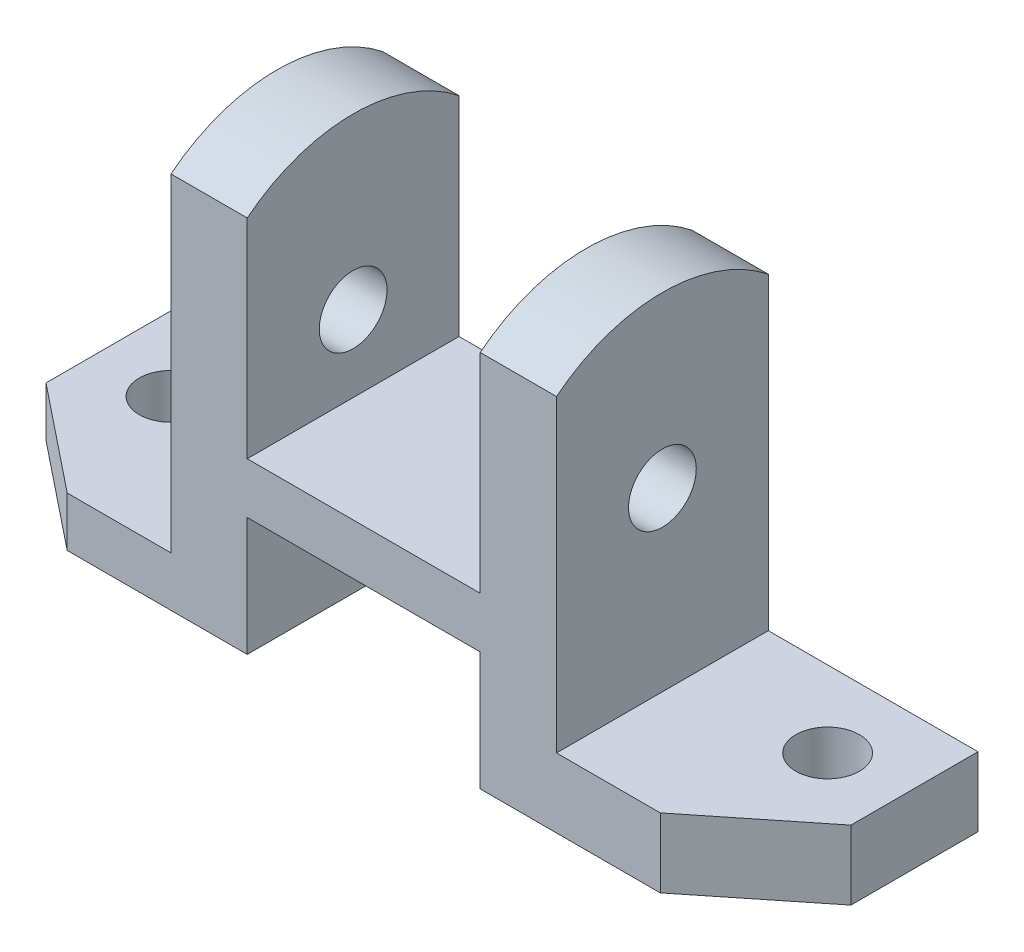
ISO-10303-21;
HEADER;
FILE_DESCRIPTION(('STEP AP214'),'2;1');
FILE_NAME('part.step','',(''),(''),'','','');
FILE_SCHEMA(('AUTOMOTIVE_DESIGN { 1 0 10303 214 1 1 1 1 }'));
ENDSEC;
DATA;
#1=APPLICATION_CONTEXT('core data for automotive mechanical design processes');
#2=APPLICATION_PROTOCOL_DEFINITION('international standard','automotive_design',2000,#1);
#3=PRODUCT_CONTEXT('',#1,'mechanical');
#4=PRODUCT('Part','Part','',(#3));
#5=PRODUCT_RELATED_PRODUCT_CATEGORY('part','',(#4));
#6=PRODUCT_DEFINITION_FORMATION('','',#4);
#7=PRODUCT_DEFINITION_CONTEXT('part definition',#1,'design');
#8=PRODUCT_DEFINITION('design','',#6,#7);
#9=PRODUCT_DEFINITION_SHAPE('','',#8);
#10=(LENGTH_UNIT() NAMED_UNIT(*) SI_UNIT(.MILLI.,.METRE.));
#11=(NAMED_UNIT(*) PLANE_ANGLE_UNIT() SI_UNIT($,.RADIAN.));
#12=(NAMED_UNIT(*) SI_UNIT($,.STERADIAN.) SOLID_ANGLE_UNIT());
#13=UNCERTAINTY_MEASURE_WITH_UNIT(LENGTH_MEASURE(1.E-05),#10,'distance_accuracy_value','');
#14=(GEOMETRIC_REPRESENTATION_CONTEXT(3) GLOBAL_UNCERTAINTY_ASSIGNED_CONTEXT((#13)) GLOBAL_UNIT_ASSIGNED_CONTEXT((#10,
#11,#12)) REPRESENTATION_CONTEXT('',''));
#15=CARTESIAN_POINT('',(0.,0.,0.));
#16=DIRECTION('',(0.,0.,1.));
#17=DIRECTION('',(1.,0.,0.));
#18=AXIS2_PLACEMENT_3D('',#15,#16,#17);
#19=CARTESIAN_POINT('',(45.5,-23.6422947131609,25.));
#20=DIRECTION('',(-1.,0.,0.));
#21=DIRECTION('',(0.,0.,1.));
#22=AXIS2_PLACEMENT_3D('',#19,#20,#21);
#23=PLANE('',#22);
#24=CARTESIAN_POINT('',(45.5,18.,0.));
#25=DIRECTION('',(1.,0.,0.));
#26=DIRECTION('',(0.,0.,-1.));
#27=AXIS2_PLACEMENT_3D('',#24,#25,#26);
#28=CIRCLE('',#27,8.);
#29=CARTESIAN_POINT('',(45.5,18.,-8.));
#30=VERTEX_POINT('',#29);
#31=EDGE_CURVE('E336',#30,#30,#28,.T.);
#32=ORIENTED_EDGE('',*,*,#31,.F.);
#33=EDGE_LOOP('',(#32));
#34=FACE_BOUND('',#33,.T.);
#35=CARTESIAN_POINT('',(45.5,18.,0.));
#36=DIRECTION('',(1.,0.,0.));
#37=DIRECTION('',(0.,0.,-1.));
#38=AXIS2_PLACEMENT_3D('',#35,#36,#37);
#39=CIRCLE('',#38,40.);
#40=CARTESIAN_POINT('',(45.5,49.224989991992,-25.));
#41=VERTEX_POINT('',#40);
#42=CARTESIAN_POINT('',(45.5,49.224989991992,25.));
#43=VERTEX_POINT('',#42);
#44=EDGE_CURVE('E342',#41,#43,#39,.T.);
#45=ORIENTED_EDGE('',*,*,#44,.T.);
#46=DIRECTION('',(0.,1.,0.));
#47=VECTOR('',#46,1.);
#48=CARTESIAN_POINT('',(45.5,-23.6422947131609,25.));
#49=LINE('',#48,#47);
#50=CARTESIAN_POINT('',(45.5,-23.6422947131609,25.));
#51=VERTEX_POINT('',#50);
#52=EDGE_CURVE('E311',#51,#43,#49,.T.);
#53=ORIENTED_EDGE('',*,*,#52,.F.);
#54=DIRECTION('',(0.,0.,-1.));
#55=VECTOR('',#54,1.);
#56=CARTESIAN_POINT('',(45.5,-23.6422947131609,25.));
#57=LINE('',#56,#55);
#58=CARTESIAN_POINT('',(45.5,-23.6422947131609,-25.));
#59=VERTEX_POINT('',#58);
#60=EDGE_CURVE('E249',#51,#59,#57,.T.);
#61=ORIENTED_EDGE('',*,*,#60,.T.);
#62=DIRECTION('',(0.,1.,0.));
#63=VECTOR('',#62,1.);
#64=CARTESIAN_POINT('',(45.5,-23.6422947131609,-25.));
#65=LINE('',#64,#63);
#66=EDGE_CURVE('E227',#59,#41,#65,.T.);
#67=ORIENTED_EDGE('',*,*,#66,.T.);
#68=EDGE_LOOP('',(#45,#53,#61,#67));
#69=FACE_BOUND('',#68,.T.);
#70=ADVANCED_FACE('F41',(#34,#69),#23,.F.);
#71=CARTESIAN_POINT('',(27.5,58.,25.));
#72=DIRECTION('',(1.,0.,0.));
#73=DIRECTION('',(0.,0.,-1.));
#74=AXIS2_PLACEMENT_3D('',#71,#72,#73);
#75=PLANE('',#74);
#76=CARTESIAN_POINT('',(27.5,18.,0.));
#77=DIRECTION('',(1.,0.,0.));
#78=DIRECTION('',(0.,0.,-1.));
#79=AXIS2_PLACEMENT_3D('',#76,#77,#78);
#80=CIRCLE('',#79,8.);
#81=CARTESIAN_POINT('',(27.5,18.,-8.));
#82=VERTEX_POINT('',#81);
#83=EDGE_CURVE('E325',#82,#82,#80,.T.);
#84=ORIENTED_EDGE('',*,*,#83,.T.);
#85=EDGE_LOOP('',(#84));
#86=FACE_BOUND('',#85,.T.);
#87=CARTESIAN_POINT('',(27.5,18.,0.));
#88=DIRECTION('',(1.,0.,0.));
#89=DIRECTION('',(0.,0.,-1.));
#90=AXIS2_PLACEMENT_3D('',#87,#88,#89);
#91=CIRCLE('',#90,40.);
#92=CARTESIAN_POINT('',(27.4999999999999,49.224989991992,-25.));
#93=VERTEX_POINT('',#92);
#94=CARTESIAN_POINT('',(27.4999999999999,49.224989991992,25.));
#95=VERTEX_POINT('',#94);
#96=EDGE_CURVE('E268',#93,#95,#91,.T.);
#97=ORIENTED_EDGE('',*,*,#96,.F.);
#98=DIRECTION('',(0.,-1.,0.));
#99=VECTOR('',#98,1.);
#100=CARTESIAN_POINT('',(27.5,58.,-25.));
#101=LINE('',#100,#99);
#102=CARTESIAN_POINT('',(27.5,0.,-25.));
#103=VERTEX_POINT('',#102);
#104=EDGE_CURVE('E229',#93,#103,#101,.T.);
#105=ORIENTED_EDGE('',*,*,#104,.T.);
#106=DIRECTION('',(0.,0.,-1.));
#107=VECTOR('',#106,1.);
#108=CARTESIAN_POINT('',(27.5,0.,25.));
#109=LINE('',#108,#107);
#110=CARTESIAN_POINT('',(27.5,0.,25.));
#111=VERTEX_POINT('',#110);
#112=EDGE_CURVE('E250',#111,#103,#109,.T.);
#113=ORIENTED_EDGE('',*,*,#112,.F.);
#114=DIRECTION('',(0.,-1.,0.));
#115=VECTOR('',#114,1.);
#116=CARTESIAN_POINT('',(27.5,58.,25.));
#117=LINE('',#116,#115);
#118=EDGE_CURVE('E313',#95,#111,#117,.T.);
#119=ORIENTED_EDGE('',*,*,#118,.F.);
#120=EDGE_LOOP('',(#97,#105,#113,#119));
#121=FACE_BOUND('',#120,.T.);
#122=ADVANCED_FACE('F420',(#86,#121),#75,.F.);
#123=CARTESIAN_POINT('',(-27.5,0.,25.));
#124=DIRECTION('',(-1.,0.,0.));
#125=DIRECTION('',(0.,-1.,0.));
#126=AXIS2_PLACEMENT_3D('',#123,#124,#125);
#127=PLANE('',#126);
#128=CARTESIAN_POINT('',(-27.5,18.,0.));
#129=DIRECTION('',(-1.,0.,0.));
#130=DIRECTION('',(0.,-1.,0.));
#131=AXIS2_PLACEMENT_3D('',#128,#129,#130);
#132=CIRCLE('',#131,8.);
#133=CARTESIAN_POINT('',(-27.5,18.,-8.));
#134=VERTEX_POINT('',#133);
#135=EDGE_CURVE('E270',#134,#134,#132,.T.);
#136=ORIENTED_EDGE('',*,*,#135,.T.);
#137=EDGE_LOOP('',(#136));
#138=FACE_BOUND('',#137,.T.);
#139=CARTESIAN_POINT('',(-27.5,18.,0.));
#140=DIRECTION('',(-1.,0.,0.));
#141=DIRECTION('',(0.,-1.,0.));
#142=AXIS2_PLACEMENT_3D('',#139,#140,#141);
#143=CIRCLE('',#142,40.);
#144=CARTESIAN_POINT('',(-27.5,49.224989991992,25.));
#145=VERTEX_POINT('',#144);
#146=CARTESIAN_POINT('',(-27.5,49.224989991992,-25.));
#147=VERTEX_POINT('',#146);
#148=EDGE_CURVE('E333',#145,#147,#143,.T.);
#149=ORIENTED_EDGE('',*,*,#148,.F.);
#150=DIRECTION('',(0.,1.,0.));
#151=VECTOR('',#150,1.);
#152=CARTESIAN_POINT('',(-27.5,0.,25.));
#153=LINE('',#152,#151);
#154=CARTESIAN_POINT('',(-27.5,0.,25.));
#155=VERTEX_POINT('',#154);
#156=EDGE_CURVE('E319',#155,#145,#153,.T.);
#157=ORIENTED_EDGE('',*,*,#156,.F.);
#158=DIRECTION('',(0.,0.,-1.));
#159=VECTOR('',#158,1.);
#160=CARTESIAN_POINT('',(-27.5,0.,25.));
#161=LINE('',#160,#159);
#162=CARTESIAN_POINT('',(-27.5,0.,-25.));
#163=VERTEX_POINT('',#162);
#164=EDGE_CURVE('E243',#155,#163,#161,.T.);
#165=ORIENTED_EDGE('',*,*,#164,.T.);
#166=DIRECTION('',(0.,1.,0.));
#167=VECTOR('',#166,1.);
#168=CARTESIAN_POINT('',(-27.5,0.,-25.));
#169=LINE('',#168,#167);
#170=EDGE_CURVE('E234',#163,#147,#169,.T.);
#171=ORIENTED_EDGE('',*,*,#170,.T.);
#172=EDGE_LOOP('',(#149,#157,#165,#171));
#173=FACE_BOUND('',#172,.T.);
#174=ADVANCED_FACE('F425',(#138,#173),#127,.F.);
#175=CARTESIAN_POINT('',(-45.5,58.,25.));
#176=DIRECTION('',(1.,0.,0.));
#177=DIRECTION('',(0.,1.,0.));
#178=AXIS2_PLACEMENT_3D('',#175,#176,#177);
#179=PLANE('',#178);
#180=CARTESIAN_POINT('',(-45.5,18.,0.));
#181=DIRECTION('',(1.,0.,0.));
#182=DIRECTION('',(0.,1.,0.));
#183=AXIS2_PLACEMENT_3D('',#180,#181,#182);
#184=CIRCLE('',#183,8.);
#185=CARTESIAN_POINT('',(-45.5,18.,-8.));
#186=VERTEX_POINT('',#185);
#187=EDGE_CURVE('E261',#186,#186,#184,.T.);
#188=ORIENTED_EDGE('',*,*,#187,.T.);
#189=EDGE_LOOP('',(#188));
#190=FACE_BOUND('',#189,.T.);
#191=DIRECTION('',(0.,-1.,0.));
#192=VECTOR('',#191,1.);
#193=CARTESIAN_POINT('',(-45.5,58.,25.));
#194=LINE('',#193,#192);
#195=CARTESIAN_POINT('',(-45.5,49.224989991992,25.));
#196=VERTEX_POINT('',#195);
#197=CARTESIAN_POINT('',(-45.5,-28.2452193475816,25.));
#198=VERTEX_POINT('',#197);
#199=EDGE_CURVE('E242',#196,#198,#194,.T.);
#200=ORIENTED_EDGE('',*,*,#199,.F.);
#201=CARTESIAN_POINT('',(-45.5,18.,0.));
#202=DIRECTION('',(1.,0.,0.));
#203=DIRECTION('',(0.,1.,0.));
#204=AXIS2_PLACEMENT_3D('',#201,#202,#203);
#205=CIRCLE('',#204,40.);
#206=CARTESIAN_POINT('',(-45.5,49.224989991992,-25.));
#207=VERTEX_POINT('',#206);
#208=EDGE_CURVE('E331',#207,#196,#205,.T.);
#209=ORIENTED_EDGE('',*,*,#208,.F.);
#210=DIRECTION('',(0.,-1.,0.));
#211=VECTOR('',#210,1.);
#212=CARTESIAN_POINT('',(-45.5,58.,-25.));
#213=LINE('',#212,#211);
#214=CARTESIAN_POINT('',(-45.5,-28.2452193475816,-25.));
#215=VERTEX_POINT('',#214);
#216=EDGE_CURVE('E240',#207,#215,#213,.T.);
#217=ORIENTED_EDGE('',*,*,#216,.T.);
#218=DIRECTION('',(0.,0.,-1.));
#219=VECTOR('',#218,1.);
#220=CARTESIAN_POINT('',(-45.5,-28.2452193475816,25.));
#221=LINE('',#220,#219);
#222=EDGE_CURVE('E239',#198,#215,#221,.T.);
#223=ORIENTED_EDGE('',*,*,#222,.F.);
#224=EDGE_LOOP('',(#200,#209,#217,#223));
#225=FACE_BOUND('',#224,.T.);
#226=ADVANCED_FACE('F466',(#190,#225),#179,.F.);
#227=CARTESIAN_POINT('',(0.,0.,25.));
#228=DIRECTION('',(0.,0.,1.));
#229=DIRECTION('',(1.,0.,0.));
#230=AXIS2_PLACEMENT_3D('',#227,#228,#229);
#231=PLANE('',#230);
#232=DIRECTION('',(0.,-1.,0.));
#233=VECTOR('',#232,1.);
#234=CARTESIAN_POINT('',(-27.5,-12.,25.));
#235=LINE('',#234,#233);
#236=CARTESIAN_POINT('',(-27.5,-12.,25.));
#237=VERTEX_POINT('',#236);
#238=CARTESIAN_POINT('',(-27.5,-40.,25.));
#239=VERTEX_POINT('',#238);
#240=EDGE_CURVE('E206',#237,#239,#235,.T.);
#241=ORIENTED_EDGE('',*,*,#240,.F.);
#242=DIRECTION('',(-1.,0.,0.));
#243=VECTOR('',#242,1.);
#244=CARTESIAN_POINT('',(-27.5,-12.,25.));
#245=LINE('',#244,#243);
#246=CARTESIAN_POINT('',(27.5,-12.,25.));
#247=VERTEX_POINT('',#246);
#248=EDGE_CURVE('E356',#247,#237,#245,.T.);
#249=ORIENTED_EDGE('',*,*,#248,.F.);
#250=DIRECTION('',(0.,-1.,0.));
#251=VECTOR('',#250,1.);
#252=CARTESIAN_POINT('',(27.5,-12.,25.));
#253=LINE('',#252,#251);
#254=CARTESIAN_POINT('',(27.5,-40.,25.));
#255=VERTEX_POINT('',#254);
#256=EDGE_CURVE('E367',#247,#255,#253,.T.);
#257=ORIENTED_EDGE('',*,*,#256,.T.);
#258=DIRECTION('',(1.,0.,0.));
#259=VECTOR('',#258,1.);
#260=CARTESIAN_POINT('',(-95.,-40.,25.));
#261=LINE('',#260,#259);
#262=CARTESIAN_POINT('',(69.9999999999999,-40.,25.));
#263=VERTEX_POINT('',#262);
#264=EDGE_CURVE('E296',#255,#263,#261,.T.);
#265=ORIENTED_EDGE('',*,*,#264,.T.);
#266=DIRECTION('',(0.,1.,0.));
#267=VECTOR('',#266,1.);
#268=CARTESIAN_POINT('',(69.9999999999999,-23.6422947131609,25.));
#269=LINE('',#268,#267);
#270=CARTESIAN_POINT('',(69.9999999999999,-23.6422947131609,25.));
#271=VERTEX_POINT('',#270);
#272=EDGE_CURVE('E269',#263,#271,#269,.T.);
#273=ORIENTED_EDGE('',*,*,#272,.T.);
#274=DIRECTION('',(-1.,0.,0.));
#275=VECTOR('',#274,1.);
#276=CARTESIAN_POINT('',(95.,-23.6422947131609,25.));
#277=LINE('',#276,#275);
#278=EDGE_CURVE('E289',#271,#51,#277,.T.);
#279=ORIENTED_EDGE('',*,*,#278,.T.);
#280=ORIENTED_EDGE('',*,*,#52,.T.);
#281=DIRECTION('',(1.,0.,0.));
#282=VECTOR('',#281,1.);
#283=CARTESIAN_POINT('',(-74.5,49.224989991992,25.));
#284=LINE('',#283,#282);
#285=EDGE_CURVE('E344',#95,#43,#284,.T.);
#286=ORIENTED_EDGE('',*,*,#285,.F.);
#287=ORIENTED_EDGE('',*,*,#118,.T.);
#288=DIRECTION('',(-1.,0.,0.));
#289=VECTOR('',#288,1.);
#290=CARTESIAN_POINT('',(27.5,0.,25.));
#291=LINE('',#290,#289);
#292=EDGE_CURVE('E317',#111,#155,#291,.T.);
#293=ORIENTED_EDGE('',*,*,#292,.T.);
#294=ORIENTED_EDGE('',*,*,#156,.T.);
#295=EDGE_CURVE('E340',#196,#145,#284,.T.);
#296=ORIENTED_EDGE('',*,*,#295,.F.);
#297=ORIENTED_EDGE('',*,*,#199,.T.);
#298=DIRECTION('',(-1.,0.,0.));
#299=VECTOR('',#298,1.);
#300=CARTESIAN_POINT('',(-45.5,-28.2452193475816,25.));
#301=LINE('',#300,#299);
#302=CARTESIAN_POINT('',(-69.9999999999999,-28.2452193475816,25.));
#303=VERTEX_POINT('',#302);
#304=EDGE_CURVE('E237',#198,#303,#301,.T.);
#305=ORIENTED_EDGE('',*,*,#304,.T.);
#306=DIRECTION('',(0.,-1.,0.));
#307=VECTOR('',#306,1.);
#308=CARTESIAN_POINT('',(-69.9999999999999,-40.0000000000001,25.));
#309=LINE('',#308,#307);
#310=CARTESIAN_POINT('',(-69.9999999999999,-40.,25.));
#311=VERTEX_POINT('',#310);
#312=EDGE_CURVE('E275',#303,#311,#309,.T.);
#313=ORIENTED_EDGE('',*,*,#312,.T.);
#314=EDGE_CURVE('E303',#311,#239,#261,.T.);
#315=ORIENTED_EDGE('',*,*,#314,.T.);
#316=EDGE_LOOP('',(#241,#249,#257,#265,#273,#279,#280,#286,#287,#293,#294,#296,#297,#305,#313,#315));
#317=FACE_BOUND('',#316,.T.);
#318=ADVANCED_FACE('F462',(#317),#231,.T.);
#319=CARTESIAN_POINT('',(0.,0.,-25.));
#320=DIRECTION('',(0.,0.,1.));
#321=DIRECTION('',(1.,0.,0.));
#322=AXIS2_PLACEMENT_3D('',#319,#320,#321);
#323=PLANE('',#322);
#324=DIRECTION('',(1.,0.,0.));
#325=VECTOR('',#324,1.);
#326=CARTESIAN_POINT('',(-95.,-40.,-25.));
#327=LINE('',#326,#325);
#328=CARTESIAN_POINT('',(27.5,-40.,-25.));
#329=VERTEX_POINT('',#328);
#330=CARTESIAN_POINT('',(95.,-40.,-25.));
#331=VERTEX_POINT('',#330);
#332=EDGE_CURVE('E203',#329,#331,#327,.T.);
#333=ORIENTED_EDGE('',*,*,#332,.F.);
#334=DIRECTION('',(0.,-1.,0.));
#335=VECTOR('',#334,1.);
#336=CARTESIAN_POINT('',(27.5,-12.,-25.));
#337=LINE('',#336,#335);
#338=CARTESIAN_POINT('',(27.5,-12.,-25.));
#339=VERTEX_POINT('',#338);
#340=EDGE_CURVE('E186',#339,#329,#337,.T.);
#341=ORIENTED_EDGE('',*,*,#340,.F.);
#342=DIRECTION('',(1.,0.,0.));
#343=VECTOR('',#342,1.);
#344=CARTESIAN_POINT('',(-27.5,-12.,-25.));
#345=LINE('',#344,#343);
#346=CARTESIAN_POINT('',(-27.5,-12.,-25.));
#347=VERTEX_POINT('',#346);
#348=EDGE_CURVE('E383',#347,#339,#345,.T.);
#349=ORIENTED_EDGE('',*,*,#348,.F.);
#350=DIRECTION('',(0.,-1.,0.));
#351=VECTOR('',#350,1.);
#352=CARTESIAN_POINT('',(-27.5,-12.,-25.));
#353=LINE('',#352,#351);
#354=CARTESIAN_POINT('',(-27.5,-40.,-25.));
#355=VERTEX_POINT('',#354);
#356=EDGE_CURVE('E200',#347,#355,#353,.T.);
#357=ORIENTED_EDGE('',*,*,#356,.T.);
#358=CARTESIAN_POINT('',(-95.,-40.,-25.));
#359=VERTEX_POINT('',#358);
#360=EDGE_CURVE('E213',#359,#355,#327,.T.);
#361=ORIENTED_EDGE('',*,*,#360,.F.);
#362=DIRECTION('',(0.,-1.,0.));
#363=VECTOR('',#362,1.);
#364=CARTESIAN_POINT('',(-95.,-28.2452193475816,-25.));
#365=LINE('',#364,#363);
#366=CARTESIAN_POINT('',(-95.,-28.2452193475816,-25.));
#367=VERTEX_POINT('',#366);
#368=EDGE_CURVE('E217',#367,#359,#365,.T.);
#369=ORIENTED_EDGE('',*,*,#368,.F.);
#370=DIRECTION('',(-1.,0.,0.));
#371=VECTOR('',#370,1.);
#372=CARTESIAN_POINT('',(-45.5,-28.2452193475816,-25.));
#373=LINE('',#372,#371);
#374=EDGE_CURVE('E218',#215,#367,#373,.T.);
#375=ORIENTED_EDGE('',*,*,#374,.F.);
#376=ORIENTED_EDGE('',*,*,#216,.F.);
#377=DIRECTION('',(1.,0.,0.));
#378=VECTOR('',#377,1.);
#379=CARTESIAN_POINT('',(-74.5,49.224989991992,-25.));
#380=LINE('',#379,#378);
#381=EDGE_CURVE('E262',#147,#207,#380,.F.);
#382=ORIENTED_EDGE('',*,*,#381,.F.);
#383=ORIENTED_EDGE('',*,*,#170,.F.);
#384=DIRECTION('',(-1.,0.,0.));
#385=VECTOR('',#384,1.);
#386=CARTESIAN_POINT('',(27.5,0.,-25.));
#387=LINE('',#386,#385);
#388=EDGE_CURVE('E235',#103,#163,#387,.T.);
#389=ORIENTED_EDGE('',*,*,#388,.F.);
#390=ORIENTED_EDGE('',*,*,#104,.F.);
#391=EDGE_CURVE('E264',#41,#93,#380,.F.);
#392=ORIENTED_EDGE('',*,*,#391,.F.);
#393=ORIENTED_EDGE('',*,*,#66,.F.);
#394=DIRECTION('',(-1.,0.,0.));
#395=VECTOR('',#394,1.);
#396=CARTESIAN_POINT('',(95.,-23.6422947131609,-25.));
#397=LINE('',#396,#395);
#398=CARTESIAN_POINT('',(95.,-23.6422947131609,-25.));
#399=VERTEX_POINT('',#398);
#400=EDGE_CURVE('E221',#399,#59,#397,.T.);
#401=ORIENTED_EDGE('',*,*,#400,.F.);
#402=DIRECTION('',(0.,1.,0.));
#403=VECTOR('',#402,1.);
#404=CARTESIAN_POINT('',(95.,-40.,-25.));
#405=LINE('',#404,#403);
#406=EDGE_CURVE('E211',#331,#399,#405,.T.);
#407=ORIENTED_EDGE('',*,*,#406,.F.);
#408=EDGE_LOOP('',(#333,#341,#349,#357,#361,#369,#375,#376,#382,#383,#389,#390,#392,#393,#401,#407));
#409=FACE_BOUND('',#408,.T.);
#410=ADVANCED_FACE('F212',(#409),#323,.F.);
#411=CARTESIAN_POINT('',(-45.5,-28.2452193475816,25.));
#412=DIRECTION('',(0.,-1.,0.));
#413=DIRECTION('',(1.,0.,0.));
#414=AXIS2_PLACEMENT_3D('',#411,#412,#413);
#415=PLANE('',#414);
#416=CARTESIAN_POINT('',(-77.5,-28.2452193475816,-7.));
#417=DIRECTION('',(0.,-1.,0.));
#418=DIRECTION('',(1.,0.,0.));
#419=AXIS2_PLACEMENT_3D('',#416,#417,#418);
#420=CIRCLE('',#419,7.5);
#421=CARTESIAN_POINT('',(-70.,-28.2452193475816,-7.));
#422=VERTEX_POINT('',#421);
#423=EDGE_CURVE('E345',#422,#422,#420,.T.);
#424=ORIENTED_EDGE('',*,*,#423,.T.);
#425=EDGE_LOOP('',(#424));
#426=FACE_BOUND('',#425,.T.);
#427=DIRECTION('',(0.,0.,-1.));
#428=VECTOR('',#427,1.);
#429=CARTESIAN_POINT('',(-95.,-28.2452193475816,25.));
#430=LINE('',#429,#428);
#431=CARTESIAN_POINT('',(-95.,-28.2452193475816,4.99999999999995));
#432=VERTEX_POINT('',#431);
#433=EDGE_CURVE('E256',#432,#367,#430,.T.);
#434=ORIENTED_EDGE('',*,*,#433,.F.);
#435=DIRECTION('',(0.780868809443031,0.,0.624695047554424));
#436=VECTOR('',#435,1.);
#437=CARTESIAN_POINT('',(-69.9999999999999,-28.2452193475816,25.));
#438=LINE('',#437,#436);
#439=EDGE_CURVE('E285',#432,#303,#438,.T.);
#440=ORIENTED_EDGE('',*,*,#439,.T.);
#441=ORIENTED_EDGE('',*,*,#304,.F.);
#442=ORIENTED_EDGE('',*,*,#222,.T.);
#443=ORIENTED_EDGE('',*,*,#374,.T.);
#444=EDGE_LOOP('',(#434,#440,#441,#442,#443));
#445=FACE_BOUND('',#444,.T.);
#446=ADVANCED_FACE('F439',(#426,#445),#415,.F.);
#447=CARTESIAN_POINT('',(-95.,-28.2452193475816,25.));
#448=DIRECTION('',(1.,0.,0.));
#449=DIRECTION('',(0.,1.,0.));
#450=AXIS2_PLACEMENT_3D('',#447,#448,#449);
#451=PLANE('',#450);
#452=DIRECTION('',(0.,0.,-1.));
#453=VECTOR('',#452,1.);
#454=CARTESIAN_POINT('',(-95.,-40.,25.));
#455=LINE('',#454,#453);
#456=CARTESIAN_POINT('',(-95.,-40.,4.99999999999995));
#457=VERTEX_POINT('',#456);
#458=EDGE_CURVE('E260',#457,#359,#455,.T.);
#459=ORIENTED_EDGE('',*,*,#458,.F.);
#460=DIRECTION('',(0.,1.,0.));
#461=VECTOR('',#460,1.);
#462=CARTESIAN_POINT('',(-95.,-28.2452193475816,4.99999999999995));
#463=LINE('',#462,#461);
#464=EDGE_CURVE('E278',#457,#432,#463,.T.);
#465=ORIENTED_EDGE('',*,*,#464,.T.);
#466=ORIENTED_EDGE('',*,*,#433,.T.);
#467=ORIENTED_EDGE('',*,*,#368,.T.);
#468=EDGE_LOOP('',(#459,#465,#466,#467));
#469=FACE_BOUND('',#468,.T.);
#470=ADVANCED_FACE('F436',(#469),#451,.F.);
#471=CARTESIAN_POINT('',(-95.,-40.,25.));
#472=DIRECTION('',(0.,1.,0.));
#473=DIRECTION('',(0.,0.,1.));
#474=AXIS2_PLACEMENT_3D('',#471,#472,#473);
#475=PLANE('',#474);
#476=CARTESIAN_POINT('',(-77.5,-40.,-7.));
#477=DIRECTION('',(0.,-1.,0.));
#478=DIRECTION('',(0.,0.,-1.));
#479=AXIS2_PLACEMENT_3D('',#476,#477,#478);
#480=CIRCLE('',#479,7.5);
#481=CARTESIAN_POINT('',(-77.5,-40.,-14.5));
#482=VERTEX_POINT('',#481);
#483=EDGE_CURVE('E376',#482,#482,#480,.T.);
#484=ORIENTED_EDGE('',*,*,#483,.F.);
#485=EDGE_LOOP('',(#484));
#486=FACE_BOUND('',#485,.T.);
#487=CARTESIAN_POINT('',(77.5,-40.,-7.));
#488=DIRECTION('',(0.,-1.,0.));
#489=DIRECTION('',(0.,0.,-1.));
#490=AXIS2_PLACEMENT_3D('',#487,#488,#489);
#491=CIRCLE('',#490,7.50000000000001);
#492=CARTESIAN_POINT('',(77.5,-40.,-14.5));
#493=VERTEX_POINT('',#492);
#494=EDGE_CURVE('E361',#493,#493,#491,.T.);
#495=ORIENTED_EDGE('',*,*,#494,.F.);
#496=EDGE_LOOP('',(#495));
#497=FACE_BOUND('',#496,.T.);
#498=DIRECTION('',(-1.,0.,0.));
#499=VECTOR('',#498,1.);
#500=CARTESIAN_POINT('',(-27.5,-40.,-11.));
#501=LINE('',#500,#499);
#502=CARTESIAN_POINT('',(27.5,-40.,-11.));
#503=VERTEX_POINT('',#502);
#504=CARTESIAN_POINT('',(-27.5,-40.,-11.));
#505=VERTEX_POINT('',#504);
#506=EDGE_CURVE('E210',#503,#505,#501,.T.);
#507=ORIENTED_EDGE('',*,*,#506,.F.);
#508=DIRECTION('',(0.,0.,1.));
#509=VECTOR('',#508,1.);
#510=CARTESIAN_POINT('',(27.5,-40.,-11.));
#511=LINE('',#510,#509);
#512=EDGE_CURVE('E59',#329,#503,#511,.T.);
#513=ORIENTED_EDGE('',*,*,#512,.F.);
#514=ORIENTED_EDGE('',*,*,#332,.T.);
#515=DIRECTION('',(0.,0.,-1.));
#516=VECTOR('',#515,1.);
#517=CARTESIAN_POINT('',(95.,-40.,25.));
#518=LINE('',#517,#516);
#519=CARTESIAN_POINT('',(95.,-40.,4.99999999999996));
#520=VERTEX_POINT('',#519);
#521=EDGE_CURVE('E253',#520,#331,#518,.T.);
#522=ORIENTED_EDGE('',*,*,#521,.F.);
#523=DIRECTION('',(-0.780868809443031,0.,0.624695047554424));
#524=VECTOR('',#523,1.);
#525=CARTESIAN_POINT('',(69.9999999999999,-40.,25.));
#526=LINE('',#525,#524);
#527=EDGE_CURVE('E273',#520,#263,#526,.T.);
#528=ORIENTED_EDGE('',*,*,#527,.T.);
#529=ORIENTED_EDGE('',*,*,#264,.F.);
#530=DIRECTION('',(0.,0.,1.));
#531=VECTOR('',#530,1.);
#532=CARTESIAN_POINT('',(27.5,-40.,25.));
#533=LINE('',#532,#531);
#534=CARTESIAN_POINT('',(27.5,-40.,-3.));
#535=VERTEX_POINT('',#534);
#536=EDGE_CURVE('E297',#535,#255,#533,.T.);
#537=ORIENTED_EDGE('',*,*,#536,.F.);
#538=DIRECTION('',(1.,0.,0.));
#539=VECTOR('',#538,1.);
#540=CARTESIAN_POINT('',(-27.5,-40.,-3.));
#541=LINE('',#540,#539);
#542=CARTESIAN_POINT('',(-27.5,-40.,-3.));
#543=VERTEX_POINT('',#542);
#544=EDGE_CURVE('E364',#543,#535,#541,.T.);
#545=ORIENTED_EDGE('',*,*,#544,.F.);
#546=DIRECTION('',(0.,0.,-1.));
#547=VECTOR('',#546,1.);
#548=CARTESIAN_POINT('',(-27.5,-40.,25.));
#549=LINE('',#548,#547);
#550=EDGE_CURVE('E67',#239,#543,#549,.T.);
#551=ORIENTED_EDGE('',*,*,#550,.F.);
#552=ORIENTED_EDGE('',*,*,#314,.F.);
#553=DIRECTION('',(-0.780868809443031,0.,-0.624695047554424));
#554=VECTOR('',#553,1.);
#555=CARTESIAN_POINT('',(-69.9999999999999,-40.,25.));
#556=LINE('',#555,#554);
#557=EDGE_CURVE('E279',#311,#457,#556,.T.);
#558=ORIENTED_EDGE('',*,*,#557,.T.);
#559=ORIENTED_EDGE('',*,*,#458,.T.);
#560=ORIENTED_EDGE('',*,*,#360,.T.);
#561=DIRECTION('',(0.,0.,-1.));
#562=VECTOR('',#561,1.);
#563=CARTESIAN_POINT('',(-27.5,-40.,-11.));
#564=LINE('',#563,#562);
#565=EDGE_CURVE('E377',#505,#355,#564,.T.);
#566=ORIENTED_EDGE('',*,*,#565,.F.);
#567=EDGE_LOOP('',(#507,#513,#514,#522,#528,#529,#537,#545,#551,#552,#558,#559,#560,#566));
#568=FACE_BOUND('',#567,.T.);
#569=ADVANCED_FACE('F202',(#486,#497,#568),#475,.F.);
#570=CARTESIAN_POINT('',(95.,-40.,25.));
#571=DIRECTION('',(-1.,0.,0.));
#572=DIRECTION('',(0.,0.,1.));
#573=AXIS2_PLACEMENT_3D('',#570,#571,#572);
#574=PLANE('',#573);
#575=DIRECTION('',(0.,0.,-1.));
#576=VECTOR('',#575,1.);
#577=CARTESIAN_POINT('',(95.,-23.6422947131609,25.));
#578=LINE('',#577,#576);
#579=CARTESIAN_POINT('',(95.,-23.6422947131609,4.99999999999996));
#580=VERTEX_POINT('',#579);
#581=EDGE_CURVE('E254',#580,#399,#578,.T.);
#582=ORIENTED_EDGE('',*,*,#581,.F.);
#583=DIRECTION('',(0.,-1.,0.));
#584=VECTOR('',#583,1.);
#585=CARTESIAN_POINT('',(95.,-40.,4.99999999999996));
#586=LINE('',#585,#584);
#587=EDGE_CURVE('E11',#580,#520,#586,.T.);
#588=ORIENTED_EDGE('',*,*,#587,.T.);
#589=ORIENTED_EDGE('',*,*,#521,.T.);
#590=ORIENTED_EDGE('',*,*,#406,.T.);
#591=EDGE_LOOP('',(#582,#588,#589,#590));
#592=FACE_BOUND('',#591,.T.);
#593=ADVANCED_FACE('F295',(#592),#574,.F.);
#594=CARTESIAN_POINT('',(95.,-23.6422947131609,25.));
#595=DIRECTION('',(0.,-1.,0.));
#596=DIRECTION('',(1.,0.,0.));
#597=AXIS2_PLACEMENT_3D('',#594,#595,#596);
#598=PLANE('',#597);
#599=CARTESIAN_POINT('',(77.5,-23.6422947131609,-7.));
#600=DIRECTION('',(0.,-1.,0.));
#601=DIRECTION('',(1.,0.,0.));
#602=AXIS2_PLACEMENT_3D('',#599,#600,#601);
#603=CIRCLE('',#602,7.50000000000001);
#604=CARTESIAN_POINT('',(85.,-23.6422947131609,-7.));
#605=VERTEX_POINT('',#604);
#606=EDGE_CURVE('E46',#605,#605,#603,.T.);
#607=ORIENTED_EDGE('',*,*,#606,.T.);
#608=EDGE_LOOP('',(#607));
#609=FACE_BOUND('',#608,.T.);
#610=ORIENTED_EDGE('',*,*,#278,.F.);
#611=DIRECTION('',(0.780868809443031,0.,-0.624695047554424));
#612=VECTOR('',#611,1.);
#613=CARTESIAN_POINT('',(69.9999999999999,-23.6422947131609,25.));
#614=LINE('',#613,#612);
#615=EDGE_CURVE('E51',#271,#580,#614,.T.);
#616=ORIENTED_EDGE('',*,*,#615,.T.);
#617=ORIENTED_EDGE('',*,*,#581,.T.);
#618=ORIENTED_EDGE('',*,*,#400,.T.);
#619=ORIENTED_EDGE('',*,*,#60,.F.);
#620=EDGE_LOOP('',(#610,#616,#617,#618,#619));
#621=FACE_BOUND('',#620,.T.);
#622=ADVANCED_FACE('F290',(#609,#621),#598,.F.);
#623=CARTESIAN_POINT('',(27.5,0.,25.));
#624=DIRECTION('',(0.,-1.,0.));
#625=DIRECTION('',(1.,0.,0.));
#626=AXIS2_PLACEMENT_3D('',#623,#624,#625);
#627=PLANE('',#626);
#628=ORIENTED_EDGE('',*,*,#388,.T.);
#629=ORIENTED_EDGE('',*,*,#164,.F.);
#630=ORIENTED_EDGE('',*,*,#292,.F.);
#631=ORIENTED_EDGE('',*,*,#112,.T.);
#632=EDGE_LOOP('',(#628,#629,#630,#631));
#633=FACE_BOUND('',#632,.T.);
#634=ADVANCED_FACE('F431',(#633),#627,.F.);
#635=CARTESIAN_POINT('',(-74.5,18.,0.));
#636=DIRECTION('',(1.,0.,0.));
#637=DIRECTION('',(0.,0.,-1.));
#638=AXIS2_PLACEMENT_3D('',#635,#636,#637);
#639=CYLINDRICAL_SURFACE('',#638,40.);
#640=ORIENTED_EDGE('',*,*,#148,.T.);
#641=ORIENTED_EDGE('',*,*,#381,.T.);
#642=ORIENTED_EDGE('',*,*,#208,.T.);
#643=ORIENTED_EDGE('',*,*,#295,.T.);
#644=EDGE_LOOP('',(#640,#641,#642,#643));
#645=FACE_BOUND('',#644,.T.);
#646=ADVANCED_FACE('F491',(#645),#639,.T.);
#647=ORIENTED_EDGE('',*,*,#96,.T.);
#648=ORIENTED_EDGE('',*,*,#285,.T.);
#649=ORIENTED_EDGE('',*,*,#44,.F.);
#650=ORIENTED_EDGE('',*,*,#391,.T.);
#651=EDGE_LOOP('',(#647,#648,#649,#650));
#652=FACE_BOUND('',#651,.T.);
#653=ADVANCED_FACE('F493',(#652),#639,.T.);
#654=CARTESIAN_POINT('',(-74.5,18.,0.));
#655=DIRECTION('',(1.,0.,0.));
#656=DIRECTION('',(0.,0.,-1.));
#657=AXIS2_PLACEMENT_3D('',#654,#655,#656);
#658=CYLINDRICAL_SURFACE('',#657,8.);
#659=CARTESIAN_POINT('',(-45.5,18.,-8.));
#660=CARTESIAN_POINT('',(-45.3125,18.,-8.));
#661=CARTESIAN_POINT('',(-45.125,18.,-8.));
#662=CARTESIAN_POINT('',(-44.75,18.,-8.));
#663=CARTESIAN_POINT('',(-44.5625,18.,-8.));
#664=CARTESIAN_POINT('',(-44.1875,18.,-8.));
#665=CARTESIAN_POINT('',(-44.,18.,-8.));
#666=CARTESIAN_POINT('',(-43.625,18.,-8.));
#667=CARTESIAN_POINT('',(-43.4375,18.,-8.));
#668=CARTESIAN_POINT('',(-43.0625,18.,-8.));
#669=CARTESIAN_POINT('',(-42.875,18.,-8.));
#670=CARTESIAN_POINT('',(-42.5,18.,-8.));
#671=CARTESIAN_POINT('',(-42.3125,18.,-8.));
#672=CARTESIAN_POINT('',(-41.9375,18.,-8.));
#673=CARTESIAN_POINT('',(-41.75,18.,-8.));
#674=CARTESIAN_POINT('',(-41.375,18.,-8.));
#675=CARTESIAN_POINT('',(-41.1875,18.,-8.));
#676=CARTESIAN_POINT('',(-40.8125,18.,-8.));
#677=CARTESIAN_POINT('',(-40.625,18.,-8.));
#678=CARTESIAN_POINT('',(-40.25,18.,-8.));
#679=CARTESIAN_POINT('',(-40.0625,18.,-8.));
#680=CARTESIAN_POINT('',(-39.6875,18.,-8.));
#681=CARTESIAN_POINT('',(-39.5,18.,-8.));
#682=CARTESIAN_POINT('',(-39.125,18.,-8.));
#683=CARTESIAN_POINT('',(-38.9375,18.,-8.));
#684=CARTESIAN_POINT('',(-38.5625,18.,-8.));
#685=CARTESIAN_POINT('',(-38.375,18.,-8.));
#686=CARTESIAN_POINT('',(-38.,18.,-8.));
#687=CARTESIAN_POINT('',(-37.8125,18.,-8.));
#688=CARTESIAN_POINT('',(-37.4375,18.,-8.));
#689=CARTESIAN_POINT('',(-37.25,18.,-8.));
#690=CARTESIAN_POINT('',(-36.875,18.,-8.));
#691=CARTESIAN_POINT('',(-36.6875,18.,-8.));
#692=CARTESIAN_POINT('',(-36.3125,18.,-8.));
#693=CARTESIAN_POINT('',(-36.125,18.,-8.));
#694=CARTESIAN_POINT('',(-35.75,18.,-8.));
#695=CARTESIAN_POINT('',(-35.5625,18.,-8.));
#696=CARTESIAN_POINT('',(-35.1875,18.,-8.));
#697=CARTESIAN_POINT('',(-35.,18.,-8.));
#698=CARTESIAN_POINT('',(-34.625,18.,-8.));
#699=CARTESIAN_POINT('',(-34.4375,18.,-8.));
#700=CARTESIAN_POINT('',(-34.0625,18.,-8.));
#701=CARTESIAN_POINT('',(-33.875,18.,-8.));
#702=CARTESIAN_POINT('',(-33.5,18.,-8.));
#703=CARTESIAN_POINT('',(-33.3125,18.,-8.));
#704=CARTESIAN_POINT('',(-32.9375,18.,-8.));
#705=CARTESIAN_POINT('',(-32.75,18.,-8.));
#706=CARTESIAN_POINT('',(-32.375,18.,-8.));
#707=CARTESIAN_POINT('',(-32.1875,18.,-8.));
#708=CARTESIAN_POINT('',(-31.8125,18.,-8.));
#709=CARTESIAN_POINT('',(-31.625,18.,-8.));
#710=CARTESIAN_POINT('',(-31.25,18.,-8.));
#711=CARTESIAN_POINT('',(-31.0625,18.,-8.));
#712=CARTESIAN_POINT('',(-30.6875,18.,-8.));
#713=CARTESIAN_POINT('',(-30.5,18.,-8.));
#714=CARTESIAN_POINT('',(-30.125,18.,-8.));
#715=CARTESIAN_POINT('',(-29.9375,18.,-8.));
#716=CARTESIAN_POINT('',(-29.5625,18.,-8.));
#717=CARTESIAN_POINT('',(-29.375,18.,-8.));
#718=CARTESIAN_POINT('',(-29.,18.,-8.));
#719=CARTESIAN_POINT('',(-28.8125,18.,-8.));
#720=CARTESIAN_POINT('',(-28.4375,18.,-8.));
#721=CARTESIAN_POINT('',(-28.25,18.,-8.));
#722=CARTESIAN_POINT('',(-27.875,18.,-8.));
#723=CARTESIAN_POINT('',(-27.6875,18.,-8.));
#724=CARTESIAN_POINT('',(-27.5,18.,-8.));
#725=B_SPLINE_CURVE_WITH_KNOTS('',3,(#659,#660,#661,#662,#663,#664,#665,#666,#667,#668,#669,
#670,#671,#672,#673,#674,#675,#676,#677,#678,#679,#680,#681,#682,#683,#684,#685,#686,#687,#688,
#689,#690,#691,#692,#693,#694,#695,#696,#697,#698,#699,#700,#701,#702,#703,#704,#705,#706,#707,
#708,#709,#710,#711,#712,#713,#714,#715,#716,#717,#718,#719,#720,#721,#722,#723,#724),
.UNSPECIFIED.,.F.,.F.,(4,2,2,2,2,2,2,2,2,2,2,2,2,2,2,2,2,2,2,2,2,2,2,2,2,2,2,2,2,2,2,2,4),(0.,
0.562500000000007,1.125,1.68750000000001,2.25,2.8125,3.375,3.9375,4.5,5.0625,5.62500000000001,
6.18750000000001,6.75000000000001,7.31250000000001,7.875,8.43750000000001,9.,9.56250000000001,
10.125,10.6875,11.25,11.8125,12.375,12.9375,13.5,14.0625,14.625,15.1875,15.75,16.3125,16.875,
17.4375,18.),.UNSPECIFIED.);
#726=EDGE_CURVE('BSEAM454',#186,#134,#725,.T.);
#727=ORIENTED_EDGE('',*,*,#187,.F.);
#728=ORIENTED_EDGE('',*,*,#135,.F.);
#729=ORIENTED_EDGE('',*,*,#726,.T.);
#730=ORIENTED_EDGE('',*,*,#726,.F.);
#731=EDGE_LOOP('',(#727,#729,#728,#730));
#732=FACE_BOUND('',#731,.T.);
#733=ADVANCED_FACE('F454',(#732),#658,.F.);
#734=CARTESIAN_POINT('',(45.5,18.,-8.));
#735=CARTESIAN_POINT('',(45.3125,18.,-8.));
#736=CARTESIAN_POINT('',(45.125,18.,-8.));
#737=CARTESIAN_POINT('',(44.75,18.,-8.));
#738=CARTESIAN_POINT('',(44.5625,18.,-8.));
#739=CARTESIAN_POINT('',(44.1875,18.,-8.));
#740=CARTESIAN_POINT('',(44.,18.,-8.));
#741=CARTESIAN_POINT('',(43.625,18.,-8.));
#742=CARTESIAN_POINT('',(43.4375,18.,-8.));
#743=CARTESIAN_POINT('',(43.0625,18.,-8.));
#744=CARTESIAN_POINT('',(42.875,18.,-8.));
#745=CARTESIAN_POINT('',(42.5,18.,-8.));
#746=CARTESIAN_POINT('',(42.3125,18.,-8.));
#747=CARTESIAN_POINT('',(41.9375,18.,-8.));
#748=CARTESIAN_POINT('',(41.75,18.,-8.));
#749=CARTESIAN_POINT('',(41.375,18.,-8.));
#750=CARTESIAN_POINT('',(41.1875,18.,-8.));
#751=CARTESIAN_POINT('',(40.8125,18.,-8.));
#752=CARTESIAN_POINT('',(40.625,18.,-8.));
#753=CARTESIAN_POINT('',(40.25,18.,-8.));
#754=CARTESIAN_POINT('',(40.0625,18.,-8.));
#755=CARTESIAN_POINT('',(39.6875,18.,-8.));
#756=CARTESIAN_POINT('',(39.5,18.,-8.));
#757=CARTESIAN_POINT('',(39.125,18.,-8.));
#758=CARTESIAN_POINT('',(38.9375,18.,-8.));
#759=CARTESIAN_POINT('',(38.5625,18.,-8.));
#760=CARTESIAN_POINT('',(38.375,18.,-8.));
#761=CARTESIAN_POINT('',(38.,18.,-8.));
#762=CARTESIAN_POINT('',(37.8125,18.,-8.));
#763=CARTESIAN_POINT('',(37.4375,18.,-8.));
#764=CARTESIAN_POINT('',(37.25,18.,-8.));
#765=CARTESIAN_POINT('',(36.875,18.,-8.));
#766=CARTESIAN_POINT('',(36.6875,18.,-8.));
#767=CARTESIAN_POINT('',(36.3125,18.,-8.));
#768=CARTESIAN_POINT('',(36.125,18.,-8.));
#769=CARTESIAN_POINT('',(35.75,18.,-8.));
#770=CARTESIAN_POINT('',(35.5625,18.,-8.));
#771=CARTESIAN_POINT('',(35.1875,18.,-8.));
#772=CARTESIAN_POINT('',(35.,18.,-8.));
#773=CARTESIAN_POINT('',(34.625,18.,-8.));
#774=CARTESIAN_POINT('',(34.4375,18.,-8.));
#775=CARTESIAN_POINT('',(34.0625,18.,-8.));
#776=CARTESIAN_POINT('',(33.875,18.,-8.));
#777=CARTESIAN_POINT('',(33.5,18.,-8.));
#778=CARTESIAN_POINT('',(33.3125,18.,-8.));
#779=CARTESIAN_POINT('',(32.9375,18.,-8.));
#780=CARTESIAN_POINT('',(32.75,18.,-8.));
#781=CARTESIAN_POINT('',(32.375,18.,-8.));
#782=CARTESIAN_POINT('',(32.1875,18.,-8.));
#783=CARTESIAN_POINT('',(31.8125,18.,-8.));
#784=CARTESIAN_POINT('',(31.625,18.,-8.));
#785=CARTESIAN_POINT('',(31.25,18.,-8.));
#786=CARTESIAN_POINT('',(31.0625,18.,-8.));
#787=CARTESIAN_POINT('',(30.6875,18.,-8.));
#788=CARTESIAN_POINT('',(30.5,18.,-8.));
#789=CARTESIAN_POINT('',(30.125,18.,-8.));
#790=CARTESIAN_POINT('',(29.9375,18.,-8.));
#791=CARTESIAN_POINT('',(29.5625,18.,-8.));
#792=CARTESIAN_POINT('',(29.375,18.,-8.));
#793=CARTESIAN_POINT('',(29.,18.,-8.));
#794=CARTESIAN_POINT('',(28.8125,18.,-8.));
#795=CARTESIAN_POINT('',(28.4375,18.,-8.));
#796=CARTESIAN_POINT('',(28.25,18.,-8.));
#797=CARTESIAN_POINT('',(27.875,18.,-8.));
#798=CARTESIAN_POINT('',(27.6875,18.,-8.));
#799=CARTESIAN_POINT('',(27.5,18.,-8.));
#800=B_SPLINE_CURVE_WITH_KNOTS('',3,(#734,#735,#736,#737,#738,#739,#740,#741,#742,#743,#744,
#745,#746,#747,#748,#749,#750,#751,#752,#753,#754,#755,#756,#757,#758,#759,#760,#761,#762,#763,
#764,#765,#766,#767,#768,#769,#770,#771,#772,#773,#774,#775,#776,#777,#778,#779,#780,#781,#782,
#783,#784,#785,#786,#787,#788,#789,#790,#791,#792,#793,#794,#795,#796,#797,#798,#799),
.UNSPECIFIED.,.F.,.F.,(4,2,2,2,2,2,2,2,2,2,2,2,2,2,2,2,2,2,2,2,2,2,2,2,2,2,2,2,2,2,2,2,4),(0.,
0.562499999999994,1.125,1.68750000000001,2.25,2.8125,3.375,3.93750000000001,4.5,5.0625,
5.62500000000001,6.18750000000001,6.75000000000001,7.3125,7.87500000000001,8.43750000000001,
9.00000000000001,9.5625,10.125,10.6875,11.25,11.8125,12.375,12.9375,13.5,14.0625,14.625,15.1875,
15.75,16.3125,16.875,17.4375,18.),.UNSPECIFIED.);
#801=EDGE_CURVE('BSEAM449',#30,#82,#800,.T.);
#802=ORIENTED_EDGE('',*,*,#31,.T.);
#803=ORIENTED_EDGE('',*,*,#83,.F.);
#804=ORIENTED_EDGE('',*,*,#801,.T.);
#805=ORIENTED_EDGE('',*,*,#801,.F.);
#806=EDGE_LOOP('',(#802,#804,#803,#805));
#807=FACE_BOUND('',#806,.T.);
#808=ADVANCED_FACE('F449',(#807),#658,.F.);
#809=CARTESIAN_POINT('',(-69.9999999999999,0.,25.));
#810=DIRECTION('',(-0.624695047554424,0.,0.780868809443031));
#811=DIRECTION('',(0.,1.,0.));
#812=AXIS2_PLACEMENT_3D('',#809,#810,#811);
#813=PLANE('',#812);
#814=ORIENTED_EDGE('',*,*,#439,.F.);
#815=ORIENTED_EDGE('',*,*,#464,.F.);
#816=ORIENTED_EDGE('',*,*,#557,.F.);
#817=ORIENTED_EDGE('',*,*,#312,.F.);
#818=EDGE_LOOP('',(#814,#815,#816,#817));
#819=FACE_BOUND('',#818,.T.);
#820=ADVANCED_FACE('F411',(#819),#813,.T.);
#821=CARTESIAN_POINT('',(69.9999999999999,0.,25.));
#822=DIRECTION('',(0.624695047554424,0.,0.780868809443031));
#823=DIRECTION('',(0.,-1.,0.));
#824=AXIS2_PLACEMENT_3D('',#821,#822,#823);
#825=PLANE('',#824);
#826=ORIENTED_EDGE('',*,*,#527,.F.);
#827=ORIENTED_EDGE('',*,*,#587,.F.);
#828=ORIENTED_EDGE('',*,*,#615,.F.);
#829=ORIENTED_EDGE('',*,*,#272,.F.);
#830=EDGE_LOOP('',(#826,#827,#828,#829));
#831=FACE_BOUND('',#830,.T.);
#832=ADVANCED_FACE('F42',(#831),#825,.T.);
#833=CARTESIAN_POINT('',(77.5,-12.,-7.));
#834=DIRECTION('',(0.,-1.,0.));
#835=DIRECTION('',(0.,0.,-1.));
#836=AXIS2_PLACEMENT_3D('',#833,#834,#835);
#837=CYLINDRICAL_SURFACE('',#836,7.50000000000001);
#838=ORIENTED_EDGE('',*,*,#494,.T.);
#839=EDGE_LOOP('',(#838));
#840=FACE_BOUND('',#839,.T.);
#841=ORIENTED_EDGE('',*,*,#606,.F.);
#842=EDGE_LOOP('',(#841));
#843=FACE_BOUND('',#842,.T.);
#844=ADVANCED_FACE('F405',(#840,#843),#837,.F.);
#845=CARTESIAN_POINT('',(-27.5,-12.,25.));
#846=DIRECTION('',(-1.,0.,0.));
#847=DIRECTION('',(0.,0.,1.));
#848=AXIS2_PLACEMENT_3D('',#845,#846,#847);
#849=PLANE('',#848);
#850=ORIENTED_EDGE('',*,*,#550,.T.);
#851=DIRECTION('',(0.,-1.,0.));
#852=VECTOR('',#851,1.);
#853=CARTESIAN_POINT('',(-27.5,-12.,-3.));
#854=LINE('',#853,#852);
#855=CARTESIAN_POINT('',(-27.5,-12.,-3.));
#856=VERTEX_POINT('',#855);
#857=EDGE_CURVE('E363',#856,#543,#854,.T.);
#858=ORIENTED_EDGE('',*,*,#857,.F.);
#859=DIRECTION('',(0.,0.,-1.));
#860=VECTOR('',#859,1.);
#861=CARTESIAN_POINT('',(-27.5,-12.,25.));
#862=LINE('',#861,#860);
#863=EDGE_CURVE('E346',#237,#856,#862,.T.);
#864=ORIENTED_EDGE('',*,*,#863,.F.);
#865=ORIENTED_EDGE('',*,*,#240,.T.);
#866=EDGE_LOOP('',(#850,#858,#864,#865));
#867=FACE_BOUND('',#866,.T.);
#868=ADVANCED_FACE('F404',(#867),#849,.F.);
#869=CARTESIAN_POINT('',(27.5,-12.,25.));
#870=DIRECTION('',(1.,0.,0.));
#871=DIRECTION('',(0.,0.,-1.));
#872=AXIS2_PLACEMENT_3D('',#869,#870,#871);
#873=PLANE('',#872);
#874=ORIENTED_EDGE('',*,*,#536,.T.);
#875=ORIENTED_EDGE('',*,*,#256,.F.);
#876=DIRECTION('',(0.,0.,1.));
#877=VECTOR('',#876,1.);
#878=CARTESIAN_POINT('',(27.5,-12.,25.));
#879=LINE('',#878,#877);
#880=CARTESIAN_POINT('',(27.5,-12.,-3.));
#881=VERTEX_POINT('',#880);
#882=EDGE_CURVE('E351',#881,#247,#879,.T.);
#883=ORIENTED_EDGE('',*,*,#882,.F.);
#884=DIRECTION('',(0.,-1.,0.));
#885=VECTOR('',#884,1.);
#886=CARTESIAN_POINT('',(27.5,-12.,-3.));
#887=LINE('',#886,#885);
#888=EDGE_CURVE('E371',#881,#535,#887,.T.);
#889=ORIENTED_EDGE('',*,*,#888,.T.);
#890=EDGE_LOOP('',(#874,#875,#883,#889));
#891=FACE_BOUND('',#890,.T.);
#892=ADVANCED_FACE('F412',(#891),#873,.F.);
#893=CARTESIAN_POINT('',(-27.5,-12.,-3.));
#894=DIRECTION('',(0.,0.,-1.));
#895=DIRECTION('',(-1.,0.,0.));
#896=AXIS2_PLACEMENT_3D('',#893,#894,#895);
#897=PLANE('',#896);
#898=ORIENTED_EDGE('',*,*,#544,.T.);
#899=ORIENTED_EDGE('',*,*,#888,.F.);
#900=DIRECTION('',(1.,0.,0.));
#901=VECTOR('',#900,1.);
#902=CARTESIAN_POINT('',(-27.5,-12.,-3.));
#903=LINE('',#902,#901);
#904=EDGE_CURVE('E355',#856,#881,#903,.T.);
#905=ORIENTED_EDGE('',*,*,#904,.F.);
#906=ORIENTED_EDGE('',*,*,#857,.T.);
#907=EDGE_LOOP('',(#898,#899,#905,#906));
#908=FACE_BOUND('',#907,.T.);
#909=ADVANCED_FACE('F482',(#908),#897,.F.);
#910=CARTESIAN_POINT('',(0.,-12.,0.));
#911=DIRECTION('',(0.,-1.,0.));
#912=DIRECTION('',(0.,0.,-1.));
#913=AXIS2_PLACEMENT_3D('',#910,#911,#912);
#914=PLANE('',#913);
#915=ORIENTED_EDGE('',*,*,#863,.T.);
#916=ORIENTED_EDGE('',*,*,#904,.T.);
#917=ORIENTED_EDGE('',*,*,#882,.T.);
#918=ORIENTED_EDGE('',*,*,#248,.T.);
#919=EDGE_LOOP('',(#915,#916,#917,#918));
#920=FACE_BOUND('',#919,.T.);
#921=ADVANCED_FACE('F480',(#920),#914,.T.);
#922=CARTESIAN_POINT('',(27.5,-12.,-11.));
#923=DIRECTION('',(1.,0.,0.));
#924=DIRECTION('',(0.,0.,-1.));
#925=AXIS2_PLACEMENT_3D('',#922,#923,#924);
#926=PLANE('',#925);
#927=ORIENTED_EDGE('',*,*,#512,.T.);
#928=DIRECTION('',(0.,-1.,0.));
#929=VECTOR('',#928,1.);
#930=CARTESIAN_POINT('',(27.5,-12.,-11.));
#931=LINE('',#930,#929);
#932=CARTESIAN_POINT('',(27.5,-12.,-11.));
#933=VERTEX_POINT('',#932);
#934=EDGE_CURVE('E387',#933,#503,#931,.T.);
#935=ORIENTED_EDGE('',*,*,#934,.F.);
#936=DIRECTION('',(0.,0.,1.));
#937=VECTOR('',#936,1.);
#938=CARTESIAN_POINT('',(27.5,-12.,-11.));
#939=LINE('',#938,#937);
#940=EDGE_CURVE('E195',#339,#933,#939,.T.);
#941=ORIENTED_EDGE('',*,*,#940,.F.);
#942=ORIENTED_EDGE('',*,*,#340,.T.);
#943=EDGE_LOOP('',(#927,#935,#941,#942));
#944=FACE_BOUND('',#943,.T.);
#945=ADVANCED_FACE('F188',(#944),#926,.F.);
#946=CARTESIAN_POINT('',(-27.5,-12.,-11.));
#947=DIRECTION('',(-1.,0.,0.));
#948=DIRECTION('',(0.,0.,1.));
#949=AXIS2_PLACEMENT_3D('',#946,#947,#948);
#950=PLANE('',#949);
#951=ORIENTED_EDGE('',*,*,#565,.T.);
#952=ORIENTED_EDGE('',*,*,#356,.F.);
#953=DIRECTION('',(0.,0.,-1.));
#954=VECTOR('',#953,1.);
#955=CARTESIAN_POINT('',(-27.5,-12.,-11.));
#956=LINE('',#955,#954);
#957=CARTESIAN_POINT('',(-27.5,-12.,-11.));
#958=VERTEX_POINT('',#957);
#959=EDGE_CURVE('E385',#958,#347,#956,.T.);
#960=ORIENTED_EDGE('',*,*,#959,.F.);
#961=DIRECTION('',(0.,-1.,0.));
#962=VECTOR('',#961,1.);
#963=CARTESIAN_POINT('',(-27.5,-12.,-11.));
#964=LINE('',#963,#962);
#965=EDGE_CURVE('E395',#958,#505,#964,.T.);
#966=ORIENTED_EDGE('',*,*,#965,.T.);
#967=EDGE_LOOP('',(#951,#952,#960,#966));
#968=FACE_BOUND('',#967,.T.);
#969=ADVANCED_FACE('F646',(#968),#950,.F.);
#970=CARTESIAN_POINT('',(-27.5,-12.,-11.));
#971=DIRECTION('',(0.,0.,1.));
#972=DIRECTION('',(1.,0.,0.));
#973=AXIS2_PLACEMENT_3D('',#970,#971,#972);
#974=PLANE('',#973);
#975=ORIENTED_EDGE('',*,*,#506,.T.);
#976=ORIENTED_EDGE('',*,*,#965,.F.);
#977=DIRECTION('',(-1.,0.,0.));
#978=VECTOR('',#977,1.);
#979=CARTESIAN_POINT('',(-27.5,-12.,-11.));
#980=LINE('',#979,#978);
#981=EDGE_CURVE('E378',#933,#958,#980,.T.);
#982=ORIENTED_EDGE('',*,*,#981,.F.);
#983=ORIENTED_EDGE('',*,*,#934,.T.);
#984=EDGE_LOOP('',(#975,#976,#982,#983));
#985=FACE_BOUND('',#984,.T.);
#986=ADVANCED_FACE('F660',(#985),#974,.F.);
#987=CARTESIAN_POINT('',(0.,-12.,0.));
#988=DIRECTION('',(0.,-1.,0.));
#989=DIRECTION('',(0.,0.,-1.));
#990=AXIS2_PLACEMENT_3D('',#987,#988,#989);
#991=PLANE('',#990);
#992=ORIENTED_EDGE('',*,*,#940,.T.);
#993=ORIENTED_EDGE('',*,*,#981,.T.);
#994=ORIENTED_EDGE('',*,*,#959,.T.);
#995=ORIENTED_EDGE('',*,*,#348,.T.);
#996=EDGE_LOOP('',(#992,#993,#994,#995));
#997=FACE_BOUND('',#996,.T.);
#998=ADVANCED_FACE('F667',(#997),#991,.T.);
#999=CARTESIAN_POINT('',(-77.5,-12.,-7.));
#1000=DIRECTION('',(0.,-1.,0.));
#1001=DIRECTION('',(0.,0.,-1.));
#1002=AXIS2_PLACEMENT_3D('',#999,#1000,#1001);
#1003=CYLINDRICAL_SURFACE('',#1002,7.5);
#1004=ORIENTED_EDGE('',*,*,#483,.T.);
#1005=EDGE_LOOP('',(#1004));
#1006=FACE_BOUND('',#1005,.T.);
#1007=ORIENTED_EDGE('',*,*,#423,.F.);
#1008=EDGE_LOOP('',(#1007));
#1009=FACE_BOUND('',#1008,.T.);
#1010=ADVANCED_FACE('F673',(#1006,#1009),#1003,.F.);
#1011=CLOSED_SHELL('',(#70,#122,#174,#226,#318,#410,#446,#470,#569,#593,#622,#634,#646,#653,
#733,#808,#820,#832,#844,#868,#892,#909,#921,#945,#969,#986,#998,#1010));
#1012=MANIFOLD_SOLID_BREP('B2',#1011);
#1013=ADVANCED_BREP_SHAPE_REPRESENTATION('',(#18,#1012),#14);
#1014=SHAPE_DEFINITION_REPRESENTATION(#9,#1013);
ENDSEC;
END-ISO-10303-21;
